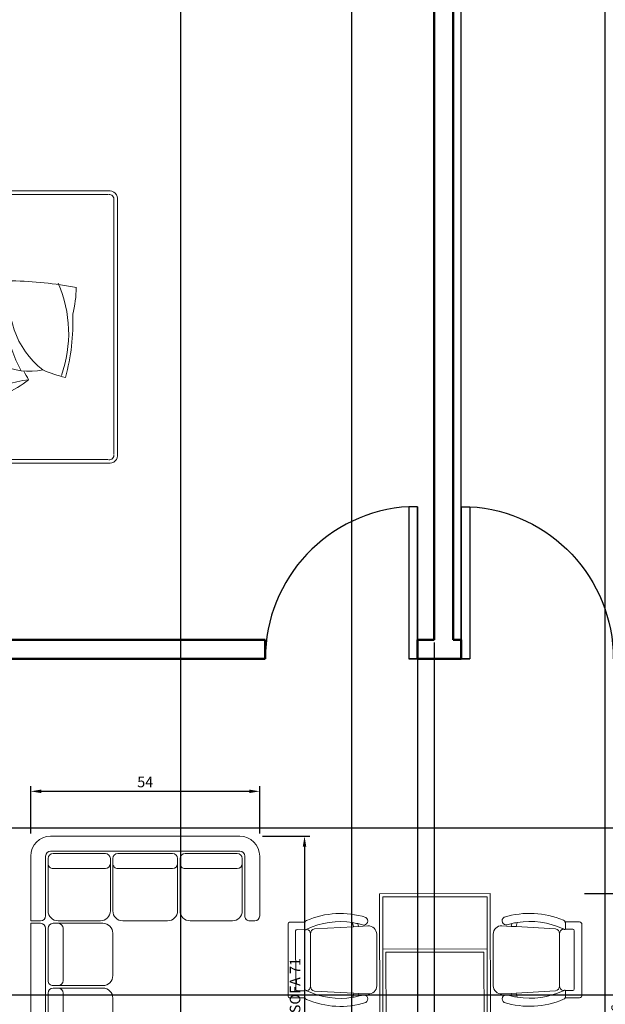
# Model space of a CAD drawing. Units: inches. Extents: x 907 to 2409, y 377 to 1163.
# Tile 5 of 9: x 1058 to 1197, y 687 to 920. Entities that reach past the tile are written whole.
import ezdxf

# ---------------------------------------------------------------- set-up
doc = ezdxf.new("R2010")
doc.units = ezdxf.units.IN
for name, color, linetype, lineweight in [('A-ANNO-DIMS', 2, 'Continuous', 18), ('A-DOOR', 3, 'Continuous', 25), ('A-FURN', 8, 'Continuous', 18), ('A-WALL', 7, 'Continuous', 50)]:
    doc.layers.add(name, color=color, linetype=linetype, lineweight=lineweight)
doc.styles.get("Standard").update_dxf_attribs({"font": 'arial.ttf'})
doc.dimstyles.new('ISO-25', dxfattribs={"dimtxt": 2.5, "dimasz": 2.5, "dimexe": 1.25, "dimexo": 0.625, "dimtad": 1, "dimtxsty": 'Standard', "dimcen": 2.5, "dimadec": 0, "dimazin": 0, "dimtfac": 1, "dimtmove": 0, "dimatfit": 3, "dimfxl": 1, "dimarcsym": 0})

# ---------------------------------------------------------------- blocks, each defined once
blk = doc.blocks.new('A$C356F0359')
for p, q in [((0.4398, 1.9801), (0.0598, 1.9801)), ((0.4398, 1.9601), (0.0598, 1.9601)), ((0.5489, 2), (2.0492, 2)), ((0.5489, 1.9489), (0.5489, 2)), ((2.0492, 1.9489), (2.0492, 2)), ((2.5283, 1.9801), (2.1483, 1.9801)), ((2.5283, 1.9601), (2.1483, 1.9601)), ((-0.0002, 1.9201), (-0.0002, 1.5401)), ((0.0198, 1.9201), (0.0198, 1.5401)), ((0.4798, 1.5401), (0.4798, 1.9201)), ((0.4998, 1.5401), (0.4998, 1.9201)), ((2.0492, 1.9489), (0.5489, 1.9489)), ((1.998, 1.9289), (0.6001, 1.9289)), ((2.0883, 1.9201), (2.0883, 1.5401)), ((2.1083, 1.9201), (2.1083, 1.5401)), ((2.5683, 1.5401), (2.5683, 1.9201)), ((2.5883, 1.5401), (2.5883, 1.9201)), ((0.1539, 1.5681), (0.1539, 1.8777)), ((0.2725, 1.8879), (0.2702, 1.8856)), ((0.2702, 1.8856), (0.2702, 1.7279)), ((0.2725, 1.8879), (0.4531, 1.8879)), ((0.3913, 1.8753), (0.277, 1.8753)), ((0.277, 1.8753), (0.277, 1.8147)), ((0.3913, 1.8147), (0.3913, 1.8753)), ((0.4016, 1.8787), (0.4062, 1.8845)), ((0.4016, 1.7404), (0.4016, 1.8787)), ((0.4062, 1.881), (0.405, 1.8765)), ((0.405, 1.8765), (0.4153, 1.8662)), ((0.405, 1.8765), (0.405, 1.8456)), ((0.405, 1.8456), (0.4073, 1.8399)), ((0.4062, 1.8845), (0.4405, 1.8845)), ((0.4108, 1.8833), (0.4062, 1.881)), ((0.4108, 1.8833), (0.4382, 1.8833)), ((0.4165, 1.8685), (0.4108, 1.8833)), ((0.4153, 1.8662), (0.4165, 1.8685)), ((0.4153, 1.8147), (0.4153, 1.8662)), ((0.4325, 1.8685), (0.4165, 1.8685)), ((0.4325, 1.8685), (0.4382, 1.8833)), ((0.4336, 1.8662), (0.4325, 1.8685)), ((0.4439, 1.8765), (0.4336, 1.8662)), ((0.4336, 1.8147), (0.4336, 1.8662)), ((0.4382, 1.8833), (0.4428, 1.881)), ((0.4405, 1.8845), (0.4462, 1.8787)), ((0.4439, 1.8456), (0.4416, 1.8399)), ((0.4428, 1.881), (0.4439, 1.8765)), ((0.4439, 1.8765), (0.4439, 1.8456)), ((0.4462, 1.8787), (0.4462, 1.7416)), ((0.4531, 1.8879), (0.4553, 1.8856)), ((0.4553, 1.8856), (0.4553, 1.7279)), ((0.5489, 1.8977), (0.5489, 0.0512)), ((0.5689, 1.8977), (0.5689, 0.0512)), ((2.0292, 0.0512), (2.0292, 1.8977)), ((2.0492, 0.0512), (2.0492, 1.8977)), ((2.3306, 1.5822), (2.3306, 1.8917)), ((0.277, 1.8147), (0.3913, 1.8147)), ((0.3913, 1.8125), (0.2816, 1.8125)), ((0.2816, 1.8125), (0.2816, 1.801)), ((0.2816, 1.801), (0.3913, 1.801)), ((0.2907, 1.8125), (0.2907, 1.801)), ((0.2999, 1.8125), (0.2999, 1.801)), ((0.309, 1.8125), (0.309, 1.801)), ((0.3182, 1.8125), (0.3182, 1.801)), ((0.3273, 1.8125), (0.3273, 1.801)), ((0.3365, 1.8125), (0.3365, 1.801)), ((0.3913, 1.801), (0.3913, 1.8125)), ((0.4073, 1.8399), (0.4108, 1.8342)), ((0.4108, 1.8342), (0.4119, 1.8262)), ((0.4108, 1.785), (0.4119, 1.793)), ((0.4119, 1.8262), (0.4119, 1.8147)), ((0.4119, 1.793), (0.4119, 1.8147)), ((0.4153, 1.8147), (0.4153, 1.753)), ((0.4336, 1.8147), (0.4336, 1.753)), ((0.4382, 1.8342), (0.4371, 1.8262)), ((0.4371, 1.8262), (0.4371, 1.8147)), ((0.4371, 1.793), (0.4371, 1.8147)), ((0.4382, 1.785), (0.4371, 1.793)), ((0.4416, 1.8399), (0.4382, 1.8342)), ((0.277, 1.7885), (0.277, 1.7679)), ((0.3445, 1.7885), (0.277, 1.7885)), ((0.277, 1.7679), (0.3445, 1.7679)), ((0.2782, 1.7622), (0.2782, 1.7576)), ((0.2896, 1.7622), (0.2782, 1.7622)), ((0.2782, 1.7576), (0.2896, 1.7576)), ((0.2782, 1.745), (0.2896, 1.745)), ((0.2782, 1.7382), (0.2782, 1.745)), ((0.2896, 1.7382), (0.2782, 1.7382)), ((0.2885, 1.7862), (0.2885, 1.7827)), ((0.2919, 1.7862), (0.2885, 1.7862)), ((0.2885, 1.7827), (0.2919, 1.7827)), ((0.2919, 1.7736), (0.2885, 1.7736)), ((0.2885, 1.7736), (0.2885, 1.7702)), ((0.2885, 1.7702), (0.2919, 1.7702)), ((0.2896, 1.7576), (0.2896, 1.7622)), ((0.2896, 1.745), (0.2896, 1.7382)), ((0.2919, 1.7827), (0.2919, 1.7862)), ((0.2919, 1.7702), (0.2919, 1.7736)), ((0.2942, 1.7622), (0.2942, 1.7576)), ((0.3056, 1.7622), (0.2942, 1.7622)), ((0.2942, 1.7576), (0.3056, 1.7576)), ((0.2942, 1.745), (0.3056, 1.745)), ((0.2942, 1.7382), (0.2942, 1.745)), ((0.3056, 1.7382), (0.2942, 1.7382)), ((0.3056, 1.7576), (0.3056, 1.7622)), ((0.3056, 1.745), (0.3056, 1.7382)), ((0.3125, 1.7862), (0.309, 1.7862)), ((0.309, 1.7862), (0.309, 1.7827)), ((0.309, 1.7827), (0.3125, 1.7827)), ((0.3125, 1.7736), (0.309, 1.7736)), ((0.309, 1.7736), (0.309, 1.7702)), ((0.309, 1.7702), (0.3125, 1.7702)), ((0.3102, 1.7622), (0.3102, 1.7576)), ((0.3216, 1.7622), (0.3102, 1.7622)), ((0.3102, 1.7576), (0.3216, 1.7576)), ((0.3102, 1.745), (0.3216, 1.745)), ((0.3102, 1.7382), (0.3102, 1.745)), ((0.3216, 1.7382), (0.3102, 1.7382)), ((0.3125, 1.7827), (0.3125, 1.7862)), ((0.3125, 1.7702), (0.3125, 1.7736)), ((0.3216, 1.7576), (0.3216, 1.7622)), ((0.3216, 1.745), (0.3216, 1.7382)), ((0.3376, 1.7622), (0.3262, 1.7622)), ((0.3262, 1.7622), (0.3262, 1.7576)), ((0.3262, 1.7576), (0.3376, 1.7576)), ((0.3262, 1.7382), (0.3262, 1.745)), ((0.3262, 1.745), (0.3376, 1.745)), ((0.3376, 1.7382), (0.3262, 1.7382)), ((0.333, 1.7862), (0.3296, 1.7862)), ((0.3296, 1.7862), (0.3296, 1.7827)), ((0.3296, 1.7827), (0.333, 1.7827)), ((0.333, 1.7736), (0.3296, 1.7736)), ((0.3296, 1.7736), (0.3296, 1.7702)), ((0.3296, 1.7702), (0.333, 1.7702)), ((0.333, 1.7827), (0.333, 1.7862)), ((0.333, 1.7702), (0.333, 1.7736)), ((0.3376, 1.7576), (0.3376, 1.7622)), ((0.3376, 1.745), (0.3376, 1.7382)), ((0.3445, 1.7679), (0.3445, 1.7885)), ((0.3548, 1.7759), (0.3548, 1.7827)), ((0.3548, 1.7827), (0.3639, 1.7827)), ((0.3639, 1.7759), (0.3548, 1.7759)), ((0.3548, 1.7633), (0.3548, 1.7702)), ((0.3548, 1.7702), (0.3639, 1.7702)), ((0.3639, 1.7633), (0.3548, 1.7633)), ((0.3548, 1.7564), (0.3639, 1.7564)), ((0.3548, 1.7496), (0.3548, 1.7564)), ((0.3639, 1.7496), (0.3548, 1.7496)), ((0.3548, 1.737), (0.3548, 1.7439)), ((0.3548, 1.7439), (0.3639, 1.7439)), ((0.3639, 1.737), (0.3548, 1.737)), ((0.3639, 1.7827), (0.3639, 1.7759)), ((0.3639, 1.7702), (0.3639, 1.7633)), ((0.3639, 1.7564), (0.3639, 1.7496)), ((0.3639, 1.7439), (0.3639, 1.737)), ((0.3685, 1.7827), (0.3776, 1.7827)), ((0.3685, 1.7759), (0.3685, 1.7827)), ((0.3776, 1.7759), (0.3685, 1.7759)), ((0.3685, 1.7633), (0.3685, 1.7702)), ((0.3685, 1.7702), (0.3776, 1.7702)), ((0.3776, 1.7633), (0.3685, 1.7633)), ((0.3685, 1.7564), (0.3776, 1.7564)), ((0.3685, 1.7496), (0.3685, 1.7564)), ((0.3776, 1.7496), (0.3685, 1.7496)), ((0.3685, 1.737), (0.3685, 1.7439)), ((0.3685, 1.7439), (0.3776, 1.7439)), ((0.3776, 1.737), (0.3685, 1.737)), ((0.3776, 1.7827), (0.3776, 1.7759)), ((0.3776, 1.7702), (0.3776, 1.7633)), ((0.3776, 1.7564), (0.3776, 1.7496)), ((0.3776, 1.7439), (0.3776, 1.737)), ((0.3822, 1.7759), (0.3822, 1.7827)), ((0.3822, 1.7827), (0.3913, 1.7827)), ((0.3913, 1.7759), (0.3822, 1.7759)), ((0.3822, 1.7633), (0.3822, 1.7702)), ((0.3822, 1.7702), (0.3913, 1.7702)), ((0.3913, 1.7633), (0.3822, 1.7633)), ((0.3822, 1.7576), (0.3913, 1.7576)), ((0.3822, 1.7507), (0.3822, 1.7576)), ((0.3913, 1.7507), (0.3822, 1.7507)), ((0.3822, 1.7439), (0.3913, 1.7439)), ((0.3822, 1.737), (0.3822, 1.7439)), ((0.3913, 1.737), (0.3822, 1.737)), ((0.3913, 1.7827), (0.3913, 1.7759)), ((0.3913, 1.7702), (0.3913, 1.7633)), ((0.3913, 1.7576), (0.3913, 1.7507)), ((0.3913, 1.7439), (0.3913, 1.737)), ((0.4073, 1.7347), (0.4016, 1.7404)), ((0.405, 1.7736), (0.4073, 1.7793)), ((0.405, 1.7427), (0.405, 1.7736)), ((0.405, 1.7427), (0.4153, 1.753)), ((0.4062, 1.7382), (0.405, 1.7427)), ((0.4108, 1.7359), (0.4062, 1.7382)), ((0.4073, 1.7793), (0.4108, 1.785)), ((0.4165, 1.7507), (0.4108, 1.7359)), ((0.4108, 1.7359), (0.4234, 1.7359)), ((0.4153, 1.753), (0.4165, 1.7507)), ((0.4325, 1.7507), (0.4165, 1.7507)), ((0.4233, 1.7393), (0.4235, 1.7294)), ((0.4268, 1.7393), (0.4233, 1.7393)), ((0.4274, 1.7301), (0.4268, 1.7393)), ((0.427, 1.7359), (0.4382, 1.7359)), ((0.4336, 1.753), (0.4325, 1.7507)), ((0.4325, 1.7507), (0.4382, 1.7359)), ((0.4439, 1.7427), (0.4336, 1.753)), ((0.4416, 1.7793), (0.4382, 1.785)), ((0.4382, 1.7359), (0.4428, 1.7382)), ((0.4462, 1.7416), (0.4405, 1.7347)), ((0.4439, 1.7736), (0.4416, 1.7793)), ((0.4428, 1.7382), (0.4439, 1.7427)), ((0.4439, 1.7427), (0.4439, 1.7736)), ((0.4622, 1.7459), (0.4553, 1.7484)), ((0.4553, 1.7439), (0.4604, 1.7425)), ((0.4604, 1.7425), (0.465, 1.7388)), ((0.4654, 1.7427), (0.4622, 1.7459)), ((0.465, 1.7388), (0.4662, 1.7372)), ((0.4678, 1.7405), (0.4654, 1.7427)), ((0.4662, 1.7372), (0.4686, 1.7374)), ((0.4686, 1.7374), (0.4662, 1.735)), ((0.4721, 1.7421), (0.4678, 1.7405)), ((0.4741, 1.7401), (0.4721, 1.7421)), ((0.4725, 1.7366), (0.4741, 1.7401)), ((0.4753, 1.7388), (0.4725, 1.7366)), ((0.4783, 1.7356), (0.4753, 1.7388)), ((2.4819, 1.7366), (2.1818, 1.7366)), ((0.3052, 1.7226), (0.0051, 1.7226)), ((0.2702, 1.7279), (0.2725, 1.7256)), ((0.4244, 1.7256), (0.2725, 1.7256)), ((0.4234, 1.7347), (0.4073, 1.7347)), ((0.4235, 1.7294), (0.4263, 1.7179)), ((0.4263, 1.7179), (0.429, 1.707)), ((0.427, 1.697), (0.4265, 1.6915)), ((0.4265, 1.6915), (0.4332, 1.6903)), ((0.4332, 1.6903), (0.4267, 1.6864)), ((0.4267, 1.6864), (0.4272, 1.6801)), ((0.4295, 1.6996), (0.427, 1.697)), ((0.4405, 1.7347), (0.4271, 1.7347)), ((0.429, 1.7227), (0.4274, 1.7301)), ((0.4531, 1.7256), (0.4284, 1.7256)), ((0.429, 1.707), (0.4288, 1.701)), ((0.4288, 1.701), (0.4295, 1.6996)), ((0.4318, 1.7119), (0.429, 1.7227)), ((0.4325, 1.7063), (0.4318, 1.7119)), ((0.4323, 1.7003), (0.4325, 1.7063)), ((0.4364, 1.6973), (0.4323, 1.7003)), ((0.4355, 1.6919), (0.4364, 1.6973)), ((0.4367, 1.6774), (0.4355, 1.6919)), ((0.4553, 1.7279), (0.4531, 1.7256)), ((0.4662, 1.735), (0.4755, 1.7268)), ((0.4755, 1.7268), (0.4906, 1.7139)), ((0.4759, 1.729), (0.4783, 1.7356)), ((0.4821, 1.7322), (0.4759, 1.729)), ((0.4874, 1.7272), (0.4821, 1.7322)), ((0.4862, 1.7199), (0.4874, 1.7272)), ((0.4914, 1.7231), (0.4862, 1.7199)), ((0.4908, 1.7135), (0.4984, 1.6917)), ((0.4958, 1.7185), (0.4914, 1.7231)), ((0.494, 1.7135), (0.4958, 1.7185)), ((0.501, 1.7142), (0.494, 1.7135)), ((0.4984, 1.6917), (0.4952, 1.6744)), ((0.4964, 1.7047), (0.5031, 1.7072)), ((0.5038, 1.7049), (0.4964, 1.7047)), ((0.5005, 1.695), (0.5054, 1.6996)), ((0.5068, 1.695), (0.5005, 1.695)), ((0.5008, 1.6871), (0.5079, 1.6892)), ((0.5068, 1.6836), (0.5008, 1.6871)), ((0.5031, 1.7072), (0.501, 1.7142)), ((0.5054, 1.6996), (0.5038, 1.7049)), ((0.5058, 1.679), (0.5068, 1.6836)), ((0.5079, 1.6892), (0.5068, 1.695)), ((0.4272, 1.6801), (0.4346, 1.6794)), ((0.4346, 1.6794), (0.4281, 1.6744)), ((0.4281, 1.6744), (0.4311, 1.669)), ((0.4311, 1.669), (0.4381, 1.6704)), ((0.4381, 1.6704), (0.4348, 1.6639)), ((0.4348, 1.6639), (0.4383, 1.6598)), ((0.4455, 1.6663), (0.4367, 1.6774)), ((0.4383, 1.6598), (0.4436, 1.6637)), ((0.4436, 1.6637), (0.4427, 1.6575)), ((0.4427, 1.6575), (0.4471, 1.6547)), ((0.4577, 1.6598), (0.4455, 1.6663)), ((0.4471, 1.6547), (0.4526, 1.6593)), ((0.4526, 1.6593), (0.4519, 1.6517)), ((0.4519, 1.6517), (0.4568, 1.6503)), ((0.4568, 1.6503), (0.4598, 1.6565)), ((0.4716, 1.6586), (0.4577, 1.6598)), ((0.4598, 1.6565), (0.4626, 1.6503)), ((0.4626, 1.6503), (0.4665, 1.6498)), ((0.4665, 1.6498), (0.4681, 1.6565)), ((0.4681, 1.6565), (0.4707, 1.6491)), ((0.4707, 1.6491), (0.4751, 1.6503)), ((0.485, 1.6644), (0.4716, 1.6586)), ((0.4751, 1.6503), (0.4753, 1.6565)), ((0.4753, 1.6565), (0.4806, 1.6519)), ((0.4806, 1.6519), (0.4843, 1.6538)), ((0.4843, 1.6538), (0.4836, 1.6607)), ((0.4836, 1.6607), (0.4885, 1.6547)), ((0.4952, 1.6744), (0.485, 1.6644)), ((0.4885, 1.6547), (0.4922, 1.6579)), ((0.4922, 1.6579), (0.4894, 1.6642)), ((0.4894, 1.6642), (0.4959, 1.6614)), ((0.4957, 1.6704), (0.5024, 1.6683)), ((0.4989, 1.6642), (0.4957, 1.6704)), ((0.4959, 1.6614), (0.4989, 1.6642)), ((0.5042, 1.673), (0.4987, 1.6792)), ((0.4987, 1.6792), (0.5058, 1.679)), ((0.5024, 1.6683), (0.5042, 1.673)), ((0.0598, 1.5001), (0.4398, 1.5001)), ((0.0598, 1.4801), (0.4398, 1.4801)), ((2.1483, 1.5001), (2.5283, 1.5001)), ((2.1483, 1.4801), (2.5283, 1.4801)), ((0.6001, 0.02), (1.998, 0.02)), ((0.6001, 0), (1.998, 0))]:
    blk.add_line(p, q)
at = {"linetype": 'ByBlock'}
for p, q in [((0.6001, 1.9147), (1.282, 1.9147)), ((0.6001, 1.6759), (0.6001, 1.9147)), ((1.282, 1.9147), (1.282, 1.6759)), ((1.3161, 1.9147), (1.998, 1.9147)), ((1.3161, 1.6759), (1.3161, 1.9147)), ((1.998, 1.9147), (1.998, 1.6759)), ((1.0687, 1.6418), (0.5489, 1.6418)), ((1.282, 1.6759), (0.6001, 1.6759)), ((1.998, 1.6759), (1.3161, 1.6759)), ((1.4185, 1.5053), (0.5489, 1.5053))]:
    blk.add_line(p, q, dxfattribs=at)
for centre in [(2.3306, 1.7366), (0.1539, 1.7226)]:
    blk.add_circle(centre, 0.12, dxfattribs=at)
for centre in [(2.3306, 1.7366), (0.1539, 1.7226)]:
    blk.add_circle(centre, 0.06)
for centre, radius, start, end in [((0.0598, 1.9201), 0.06, 90, 180), ((0.0598, 1.9201), 0.04, 90, 180), ((0.4398, 1.9201), 0.06, 0, 90), ((0.4398, 1.9201), 0.04, 0, 90), ((2.1483, 1.9201), 0.06, 90, 180), ((2.1483, 1.9201), 0.04, 90, 180), ((2.5283, 1.9201), 0.06, 0, 90), ((2.5283, 1.9201), 0.04, 0, 90), ((0.6001, 1.8977), 0.0512, 90, 180), ((0.6001, 1.8977), 0.0312, 90, 180), ((1.998, 1.8977), 0.0512, 0, 90), ((1.998, 1.8977), 0.0312, 0, 90), ((0.0598, 1.5401), 0.06, 180, 270), ((0.0598, 1.5401), 0.04, 180, 270), ((0.4398, 1.5401), 0.04, 270, 0), ((0.4398, 1.5401), 0.06, 270, 0), ((2.1483, 1.5401), 0.06, 180, 270), ((2.1483, 1.5401), 0.04, 180, 270), ((2.5283, 1.5401), 0.06, 270, 0), ((2.5283, 1.5401), 0.04, 270, 0), ((1.1471, 0.7332), 0.3575, 102.4782, 140.4625), ((1.9086, 1.3124), 0.8697, 195.336, 226.4193), ((0.3249, 0.4335), 0.9879, 28.4971, 41.0566), ((0.9965, 0.4273), 0.548, 103.2034, 117.0362), ((1.6529, 1.7059), 1.0798, 223.6306, 251.4288), ((0.4451, 0.4375), 0.5655, 5.3391, 57.6895), ((0.4517, 0.5274), 0.4879, 10.6986, 52.6864), ((1.8195, 1.3719), 1.1652, 203.0642, 220.3209), ((0.5617, 0.4344), 0.7874, 18.3527, 36.6851), ((-0.021, 2.4319), 2.1977, 305.2966, 307.2418), ((1.5949, 0.9312), 0.734, 205.259, 216.9351), ((1.4135, 0.487), 0.3575, 154.0418, 192.0262), ((1.3641, 0.0041), 0.6085, 71.81, 120.1351), ((1.1372, -0.3434), 0.9879, 80.0607, 92.6202), ((1.2836, -0.1573), 0.7874, 69.9163, 88.2487), ((1.44, 0.1186), 0.4774, 76.1849, 142.0017), ((-0.6432, 0.628), 2.1977, 349.4884, 358.8054), ((-0.021, 2.4319), 2.1977, 297.9248, 299.3793), ((1.5595, 0.1789), 0.548, 154.767, 168.5998), ((1.2647, 0.9578), 0.6885, 250.2936, 293.6414), ((1.3312, 1.4107), 1.1652, 254.6278, 271.8845), ((1.5368, 0.9609), 0.734, 256.8226, 268.4988), ((0.5943, 0.0454), 0.0458, 172.7599, 277.2401), ((0.5943, 0.0454), 0.0258, 172.7599, 277.2401), ((2.0038, 0.0454), 0.0458, 262.7599, 7.2401), ((2.0038, 0.0454), 0.0258, 262.7599, 7.2401)]:
    blk.add_arc(centre, radius, start, end)
for centre, radius, start, end in [((0.1906, 1.7953), 0.4265, 343.7398, 16.2602), ((1.6914, 1.7953), 0.4265, 163.7398, 196.2602), ((0.9067, 1.7953), 0.4265, 343.7398, 16.2602), ((2.4075, 1.7953), 0.4265, 163.7398, 196.2602), ((0.9303, 0.657), 0.9853, 61.4328, 88.1261), ((1.0826, 0.5712), 1.0706, 72.1966, 90.7418), ((2.1368, 4.5996), 3.0955, 256.4201, 268.3789), ((2.0056, 2.7745), 1.3903, 244.2427, 271.7984)]:
    blk.add_arc(centre, radius, start, end, dxfattribs=at)
blk = doc.blocks.new('A$C2AFA021D')
for p, q in [((0.8, 2.3), (0.2, 2.3)), ((0.85, 2.2), (0.85, 2.25)), ((0, 2.1), (0, 0.2)), ((0.15, 0.2), (0.15, 2.1)), ((0.2, 2.15), (0.8, 2.15)), ((0.225, 2.125), (0.275, 2.125)), ((0.75, 2.125), (0.275, 2.125)), ((0.175, 1.55), (0.175, 2.075)), ((0.325, 2.075), (0.325, 1.55)), ((0.85, 1.6), (0.85, 2.025)), ((0.275, 1.5), (0.225, 1.5)), ((0.275, 1.5), (0.75, 1.5)), ((0.175, 0.875), (0.175, 1.425)), ((0.225, 1.475), (0.275, 1.475)), ((0.75, 1.475), (0.275, 1.475)), ((0.325, 1.425), (0.325, 0.875)), ((0.85, 0.925), (0.85, 1.375)), ((0.275, 0.825), (0.225, 0.825)), ((0.225, 0.8), (0.275, 0.8)), ((0.275, 0.825), (0.75, 0.825)), ((0.75, 0.8), (0.275, 0.8)), ((0.975, 0.825), (1.4, 0.825)), ((1.625, 0.825), (2.075, 0.825)), ((2.3, 0.825), (2.725, 0.825)), ((2.9, 0.825), (2.95, 0.825)), ((0.175, 0.225), (0.175, 0.75)), ((0.325, 0.75), (0.325, 0.225)), ((0.85, 0.275), (0.85, 0.7)), ((0.875, 0.275), (0.875, 0.725)), ((1.5, 0.725), (1.5, 0.275)), ((1.525, 0.275), (1.525, 0.725)), ((2.175, 0.725), (2.175, 0.275)), ((2.2, 0.275), (2.2, 0.725)), ((2.825, 0.725), (2.825, 0.275)), ((2.85, 0.2), (2.85, 0.775)), ((3, 0.775), (3, 0.2)), ((1.45, 0.325), (0.925, 0.325)), ((2.125, 0.325), (1.575, 0.325)), ((2.775, 0.325), (2.25, 0.325)), ((0.875, 0.275), (0.875, 0.225)), ((1.5, 0.225), (1.5, 0.275)), ((1.525, 0.275), (1.525, 0.225)), ((2.175, 0.225), (2.175, 0.275)), ((2.2, 0.275), (2.2, 0.225)), ((2.825, 0.225), (2.825, 0.275)), ((0.8, 0.15), (0.2, 0.15)), ((0.275, 0.175), (0.225, 0.175)), ((0.275, 0.175), (0.75, 0.175)), ((0.85, 0), (0.85, 0.1)), ((0.875, 0.1), (0.875, 0)), ((0.925, 0.175), (1.45, 0.175)), ((0.925, 0.15), (2.8, 0.15)), ((1.575, 0.175), (2.125, 0.175)), ((2.25, 0.175), (2.775, 0.175)), ((0.2, 0), (0.85, 0)), ((2.8, 0), (0.875, 0))]:
    blk.add_line(p, q)
for centre, radius, start, end in [((0.2, 2.1), 0.2, 90, 180), ((0.8, 2.25), 0.05, 0, 90), ((0.8, 2.2), 0.05, 270, 0), ((0.2, 2.1), 0.05, 90, 180), ((0.225, 2.075), 0.05, 90, 180), ((0.275, 2.075), 0.05, 0, 90), ((0.75, 2.025), 0.1, 0, 90), ((0.75, 1.6), 0.1, 270, 0), ((0.225, 1.55), 0.05, 180, 270), ((0.275, 1.55), 0.05, 270, 0), ((0.225, 1.425), 0.05, 90, 180), ((0.275, 1.425), 0.05, 0, 90), ((0.75, 1.375), 0.1, 360, 90), ((0.75, 0.925), 0.1, 270, 0), ((0.225, 0.875), 0.05, 180, 270), ((0.225, 0.75), 0.05, 90, 180), ((0.275, 0.875), 0.05, 270, 0), ((0.275, 0.75), 0.05, 0, 90), ((0.75, 0.7), 0.1, 0, 90), ((0.975, 0.725), 0.1, 90, 180), ((1.4, 0.725), 0.1, 0, 90), ((1.625, 0.725), 0.1, 90, 180), ((2.075, 0.725), 0.1, 0, 90), ((2.3, 0.725), 0.1, 90, 180), ((2.725, 0.725), 0.1, 0, 90), ((2.9, 0.775), 0.05, 90, 180), ((2.95, 0.775), 0.05, 0, 90), ((0.925, 0.275), 0.05, 90, 180), ((1.45, 0.275), 0.05, 360, 90), ((1.575, 0.275), 0.05, 90, 180), ((2.125, 0.275), 0.05, 360, 90), ((2.25, 0.275), 0.05, 90, 180), ((2.775, 0.275), 0.05, 360, 90), ((0.2, 0.2), 0.2, 180, 270), ((0.2, 0.2), 0.05, 180, 270), ((0.225, 0.225), 0.05, 180, 270), ((0.275, 0.225), 0.05, 270, 0), ((0.75, 0.275), 0.1, 270, 0), ((0.925, 0.225), 0.05, 180, 270), ((1.45, 0.225), 0.05, 270, 0), ((1.575, 0.225), 0.05, 180, 270), ((2.125, 0.225), 0.05, 270, 0), ((2.25, 0.225), 0.05, 180, 270), ((2.775, 0.225), 0.05, 270, 0), ((2.8, 0.2), 0.2, 270, 0), ((2.8, 0.2), 0.05, 270, 0), ((0.8, 0.1), 0.05, 0, 90), ((0.925, 0.1), 0.05, 90, 180)]:
    blk.add_arc(centre, radius, start, end)
blk = doc.blocks.new('A$C7D96336B')
for p, q in [((280, 0.2), (-280, -0.2)), ((280.8, -1199.8), (280, 0.2)), ((-280, -0.2), (-279.2, -1200.2)), ((264, -15.8), (-264, -16.2)), ((-264, -16.2), (-263.2, -1184.2)), ((264.8, -1183.8), (264, -15.8)), ((-658.1, -143.4), (-730.7, -143.6)), ((-659.8, -143.4), (-659.7, -178.7)), ((-416.5, -146.3), (-411.5, -167.3)), ((416.7, -145.7), (411.7, -166.7)), ((658.3, -142.5), (730.9, -142.6)), ((659.9, -142.6), (659.9, -177.8)), ((-742.8, -515.1), (-743.2, -156.2)), ((-704.9, -188.8), (-704.6, -482.3)), ((-659.3, -180.3), (-696.6, -180.5)), ((-411.5, -167.3), (-609.1, -178.7)), ((-386.1, -165.8), (-411.5, -167.3)), ((-389.5, -151.7), (-386.1, -165.8)), ((-338.9, -163.1), (-386.1, -165.8)), ((339.1, -162.6), (386.3, -165.3)), ((389.7, -151.1), (386.3, -165.3)), ((386.3, -165.3), (411.7, -166.7)), ((411.7, -166.7), (609.3, -177.8)), ((659.5, -179.5), (696.9, -179.5)), ((705.2, -187.9), (705.3, -481.4)), ((743.5, -514.1), (743.4, -155.2)), ((-629.9, -467.6), (-630.2, -203.4)), ((-294.5, -465.7), (-294.4, -204.7)), ((295.2, -465.3), (294.7, -204.3)), ((630.5, -466.8), (630.5, -202.5)), ((-263.8, -280.2), (264.2, -279.8)), ((-263.8, -280.2), (264.2, -279.8)), ((-263.4, -920.2), (-263.8, -280.2)), ((-247.8, -296.2), (248.2, -295.8)), ((-247.4, -904.2), (-247.8, -296.2)), ((248.2, -295.8), (248.6, -903.8)), ((264.2, -279.8), (264.6, -919.8)), ((-659, -490.7), (-696.3, -490.7)), ((-659.4, -522.3), (-659.3, -492.4)), ((-411.1, -503.3), (-608.7, -492.3)), ((411.8, -502.7), (609.4, -491.4)), ((659.6, -489.8), (697, -489.7)), ((660.1, -521.4), (660, -491.5)), ((-657.7, -527.6), (-730.3, -527.6)), ((-416.1, -524.3), (-411.1, -503.3)), ((-385.8, -504.7), (-411.1, -503.3)), ((-389.1, -518.8), (-385.8, -504.7)), ((-338.5, -507.3), (-385.8, -504.7)), ((339.2, -506.9), (386.5, -504.2)), ((386.5, -504.2), (411.8, -502.7)), ((389.8, -518.3), (386.5, -504.2)), ((416.8, -523.7), (411.8, -502.7)), ((658.4, -526.7), (731, -526.6)), ((-742.7, -688.4), (-742.6, -1047.3)), ((-657.6, -675.8), (-730.2, -675.9)), ((-659.3, -681), (-659.2, -711)), ((-416, -678.8), (-411, -699.8)), ((-389, -684.2), (-385.6, -698.3)), ((-338.4, -695.6), (-385.6, -698.3)), ((339.3, -695.2), (386.6, -697.8)), ((389.9, -683.7), (386.6, -697.8)), ((416.9, -678.2), (411.9, -699.2)), ((658.5, -674.9), (731.1, -674.9)), ((660.2, -680.2), (660.2, -710.1)), ((743.6, -687.4), (744, -1046.3)), ((-704.4, -1014.6), (-704.5, -721.1)), ((-658.8, -712.7), (-696.2, -712.8)), ((-629.7, -735.7), (-629.6, -1000)), ((-411, -699.8), (-608.6, -711)), ((-385.6, -698.3), (-411, -699.8)), ((-294.4, -737.1), (-293.9, -998.2)), ((295.3, -736.7), (295.2, -997.8)), ((386.6, -697.8), (411.9, -699.2)), ((411.9, -699.2), (609.5, -710.2)), ((630.7, -734.9), (631, -999.1)), ((659.8, -711.8), (697.1, -711.8)), ((705.8, -1013.7), (705.5, -720.2)), ((264.6, -919.8), (-263.4, -920.2)), ((248.6, -903.8), (-247.4, -904.2)), ((-658.7, -1023), (-696.1, -1023)), ((-659.1, -1059.9), (-659.1, -1024.7)), ((-410.9, -1035.8), (-608.5, -1024.6)), ((-415.9, -1056.8), (-410.9, -1035.8)), ((-385.5, -1037.2), (-410.9, -1035.8)), ((-388.9, -1051.4), (-385.5, -1037.2)), ((-338.3, -1039.9), (-385.5, -1037.2)), ((339.7, -1039.4), (386.9, -1036.7)), ((386.9, -1036.7), (412.3, -1035.2)), ((390.3, -1050.8), (386.9, -1036.7)), ((412.3, -1035.2), (609.9, -1023.8)), ((417.3, -1056.2), (412.3, -1035.2)), ((660.1, -1022.1), (697.4, -1022)), ((660.6, -1059), (660.5, -1023.8)), ((-657.5, -1059.9), (-730.1, -1059.9)), ((658.9, -1059), (731.5, -1058.9)), ((-263.2, -1184.2), (264.8, -1183.8)), ((-279.2, -1200.2), (280.8, -1199.8))]:
    blk.add_line(p, q)
for centre, radius, start, end in [((-730.7, -156.1), 12.5, 141.7605, 180.1459), ((-730.7, -156.1), 12.5, 90.1463, 141.7605), ((-643.2, -151), 16.7, 153.004, 184.8567), ((-643.2, -151), 16.7, 113.3258, 153.004), ((-478.6, -532.7), 432.3, 72.7119, 113.3258), ((-479.1, -531.9), 390.7, 80.7703, 115.5809), ((-479.1, -531.9), 390.7, 76.7336, 80.7703), ((-360.6, -137.9), 20.8, 254.7795, 60.0186), ((360.7, -137.4), 20.8, 120.0589, 285.298), ((479.4, -532), 432.3, 66.7517, 107.3656), ((479.9, -531.2), 390.7, 99.3072, 103.3439), ((479.9, -531.2), 390.7, 64.4966, 99.3072), ((643.4, -150.1), 16.7, 27.0735, 66.7517), ((643.4, -150.1), 16.7, 355.2209, 27.0735), ((730.9, -155.1), 12.5, 38.317, 89.9312), ((730.9, -155.1), 12.5, 359.9316, 38.317), ((-696.6, -188.8), 8.33, 90.1463, 180.1463), ((-655.5, -178.6), 4.17, 180.1463, 296.5296), ((-479.1, -531.9), 390.7, 115.5809, 116.5296), ((-655.2, -203.4), 25, 0.1463, 72.8968), ((-605.2, -203.4), 25, 98.9209, 179.9714), ((-479.1, -531.9), 390.7, 73.1676, 76.7336), ((-336.5, -204.7), 41.7, 0.1463, 93.3068), ((336.7, -204.2), 41.7, 86.7707, 179.9312), ((479.9, -531.2), 390.7, 103.3439, 106.9099), ((605.5, -202.6), 25, 0.1061, 81.1566), ((655.5, -202.5), 25, 107.1807, 179.9312), ((479.9, -531.2), 390.7, 63.5479, 64.4966), ((655.7, -177.8), 4.17, 243.5479, 359.9312), ((696.9, -187.8), 8.33, 359.9312, 89.9312), ((-696.3, -482.3), 8.33, 179.9714, 269.9714), ((-655.2, -492.4), 4.17, 63.5881, 179.9714), ((-479.5, -138.8), 390.7, 243.5881, 244.5368), ((-654.9, -467.6), 25, 287.2209, 359.9714), ((-479.5, -138.8), 390.7, 244.5368, 279.3474), ((-604.9, -467.6), 25, 180.1463, 261.1967), ((-336.2, -465.7), 41.7, 266.8108, 359.9714), ((336.8, -465.3), 41.7, 180.1061, 273.2667), ((479.7, -138.1), 390.7, 260.7301, 295.5407), ((605.5, -466.7), 25, 278.8808, 359.9312), ((655.5, -466.7), 25, 180.1061, 252.8566), ((479.7, -138.1), 390.7, 295.5407, 296.4894), ((655.8, -491.5), 4.17, 0.1061, 116.4894), ((697, -481.4), 8.33, 270.1061, 0.1061), ((-730.3, -515.1), 12.5, 179.9717, 218.3572), ((-730.3, -515.1), 12.5, 218.3572, 269.9714), ((-642.9, -520), 16.7, 175.261, 207.1136), ((-642.9, -520), 16.7, 207.1136, 246.7919), ((-479.1, -138), 432.3, 246.7919, 287.4058), ((-479.5, -138.8), 390.7, 279.3474, 283.3841), ((-479.5, -138.8), 390.7, 283.3841, 286.9501), ((-360.2, -532.5), 20.8, 300.0991, 105.3382), ((360.9, -532), 20.8, 74.7393, 239.9785), ((479.2, -137.3), 432.3, 252.6717, 293.2857), ((479.7, -138.1), 390.7, 253.1274, 256.6934), ((479.7, -138.1), 390.7, 256.6934, 260.7301), ((643.6, -519.1), 16.7, 293.2857, 332.9639), ((643.6, -519.1), 16.7, 332.9639, 4.8165), ((731, -514.1), 12.5, 270.1061, 321.7203), ((731, -514.1), 12.5, 321.7203, 0.1058), ((-478.4, -1065.1), 432.3, 72.6717, 113.2857), ((479.9, -1064.5), 432.3, 66.7919, 107.4058), ((-730.2, -688.4), 12.5, 141.7203, 180.1058), ((-730.2, -688.4), 12.5, 90.1061, 141.7203), ((-642.7, -683.3), 16.7, 152.9639, 184.8165), ((-642.7, -683.3), 16.7, 113.2857, 152.9639), ((-478.9, -1064.3), 390.7, 80.7301, 115.5407), ((-478.9, -1064.3), 390.7, 76.6934, 80.7301), ((-478.9, -1064.3), 390.7, 73.1274, 76.6934), ((-360.1, -670.4), 20.8, 254.7393, 59.9785), ((-336, -737.2), 41.7, 0.1061, 93.2667), ((337, -736.8), 41.7, 86.8108, 179.9714), ((361, -670), 20.8, 120.0991, 285.3382), ((480.4, -1063.7), 390.7, 103.3841, 106.9501), ((480.4, -1063.7), 390.7, 99.3474, 103.3841), ((480.4, -1063.7), 390.7, 64.5368, 99.3474), ((643.7, -682.5), 16.7, 27.1136, 66.7919), ((643.7, -682.5), 16.7, 355.261, 27.1136), ((731.1, -687.4), 12.5, 38.3572, 89.9714), ((731.1, -687.4), 12.5, 359.9717, 38.3572), ((-696.1, -721.1), 8.33, 90.1061, 180.1061), ((-655, -711), 4.17, 180.1061, 296.4894), ((-478.9, -1064.3), 390.7, 115.5407, 116.4894), ((-654.7, -735.8), 25, 0.1061, 72.8566), ((-604.7, -735.7), 25, 98.8808, 179.9312), ((605.7, -734.9), 25, 0.1463, 81.1967), ((655.7, -734.9), 25, 107.2209, 179.9714), ((480.4, -1063.7), 390.7, 63.5881, 64.5368), ((656, -710.1), 4.17, 243.5881, 359.9714), ((697.1, -720.1), 8.33, 359.9714, 89.9714), ((-696.1, -1014.6), 8.33, 179.9312, 269.9312), ((-654.9, -1024.7), 4.17, 63.5479, 179.9312), ((-479.1, -671.2), 390.7, 243.5479, 244.4966), ((-654.6, -1000), 25, 287.1807, 359.9312), ((-479.1, -671.2), 390.7, 244.4966, 279.3072), ((-604.6, -999.9), 25, 180.1061, 261.1566), ((-479.1, -671.2), 390.7, 283.3439, 286.9099), ((-359.9, -1065.1), 20.8, 300.0589, 105.298), ((-335.9, -998.3), 41.7, 266.7707, 359.9312), ((337.3, -997.8), 41.7, 180.1463, 273.3068), ((361.4, -1064.6), 20.8, 74.7795, 240.0186), ((480, -670.6), 390.7, 253.1676, 256.7336), ((480, -670.6), 390.7, 260.7703, 295.5809), ((606, -999.1), 25, 278.9209, 359.9714), ((656, -999.1), 25, 180.1463, 252.8968), ((480, -670.6), 390.7, 295.5809, 296.5296), ((656.3, -1023.8), 4.17, 0.1463, 116.5296), ((697.4, -1013.7), 8.33, 270.1463, 0.1463), ((-730.1, -1047.4), 12.5, 179.9316, 218.317), ((-730.1, -1047.4), 12.5, 218.317, 269.9312), ((-642.6, -1052.4), 16.7, 175.2209, 207.0735), ((-642.6, -1052.4), 16.7, 207.0735, 246.7517), ((-478.6, -670.4), 432.3, 246.7517, 287.3656), ((-479.1, -671.2), 390.7, 279.3072, 283.3439), ((479.5, -669.8), 432.3, 252.7119, 293.3258), ((480, -670.6), 390.7, 256.7336, 260.7703), ((644, -1051.5), 16.7, 293.3258, 333.004), ((644, -1051.5), 16.7, 333.004, 4.8567), ((731.5, -1046.4), 12.5, 270.1463, 321.7605), ((731.5, -1046.4), 12.5, 321.7605, 0.1459)]:
    blk.add_arc(centre, radius, start, end)
blk = doc.blocks.new('DOOR-36IN')
for p, q in [((36, 36), (36, 0)), ((36, 0), (34, 0)), ((36, 0), (34, 0))]:
    blk.add_line(p, q)
blk.add_lwpolyline([(36, 36), (34, 36), (34, 0), (36, 0)], close=True)
blk.add_arc((36.06, 0), 36.06, 93.2732, 180)
blk = doc.blocks.new('*D53')
at = {"layer": 'A-ANNO-DIMS', "color": 0, "lineweight": -2, "transparency": 16777216}
for p, q in [((1115.67, 726.66), (1126.9, 726.66)), ((1125.65, 724.16), (1125.65, 658.44)), ((1115.67, 655.94), (1126.9, 655.94))]:
    blk.add_line(p, q, dxfattribs=at)
at = {"layer": 'A-ANNO-DIMS', "color": 0, "transparency": 16777216}
for points in [[(1125.24, 724.16), (1126.07, 724.16), (1125.65, 726.66)], [(1125.24, 658.44), (1126.07, 658.44), (1125.65, 655.94)]]:
    blk.add_solid(points, dxfattribs=at)
at = {"layer": 'Defpoints', "color": 0, "transparency": 16777216}
for p in [(1115.05, 726.66), (1115.05, 655.94), (1125.65, 655.94)]:
    blk.add_point(p, dxfattribs=at)
at = {"layer": 'A-ANNO-DIMS', "color": 0, "transparency": 16777216, "insert": (1123.74, 691.3), "char_height": 2.5, "attachment_point": 5, "rotation": 90}
blk.add_mtext('SOFA 71', dxfattribs=at)
blk = doc.blocks.new('*D54')
at = {"layer": 'A-ANNO-DIMS', "color": 0, "lineweight": -2, "transparency": 16777216}
for p, q in [((1060.83, 727.28), (1060.83, 738.52)), ((1063.33, 737.27), (1112.55, 737.27)), ((1115.05, 727.28), (1115.05, 738.52))]:
    blk.add_line(p, q, dxfattribs=at)
at = {"layer": 'A-ANNO-DIMS', "color": 0, "transparency": 16777216}
for points in [[(1063.33, 737.68), (1063.33, 736.85), (1060.83, 737.27)], [(1112.55, 737.68), (1112.55, 736.85), (1115.05, 737.27)]]:
    blk.add_solid(points, dxfattribs=at)
at = {"layer": 'Defpoints', "color": 0, "transparency": 16777216}
for p in [(1115.05, 737.27), (1060.83, 726.66), (1115.05, 726.66)]:
    blk.add_point(p, dxfattribs=at)
at = {"layer": 'A-ANNO-DIMS', "color": 0, "transparency": 16777216, "insert": (1087.94, 739.16), "char_height": 2.5, "attachment_point": 5}
blk.add_mtext('54', dxfattribs=at)
blk = doc.blocks.new('*D58')
at = {"layer": 'A-ANNO-DIMS', "color": 0, "lineweight": -2, "transparency": 16777216}
for p, q in [((1191.96, 713.06), (1203.02, 713.06)), ((1201.77, 659.4), (1201.77, 710.56)), ((1191.96, 656.9), (1203.02, 656.9))]:
    blk.add_line(p, q, dxfattribs=at)
at = {"layer": 'A-ANNO-DIMS', "color": 0, "transparency": 16777216}
for points in [[(1201.36, 710.56), (1202.19, 710.56), (1201.77, 713.06)], [(1201.36, 659.4), (1202.19, 659.4), (1201.77, 656.9)]]:
    blk.add_solid(points, dxfattribs=at)
at = {"layer": 'Defpoints', "color": 0, "transparency": 16777216}
for p in [(1191.34, 713.06), (1201.77, 713.06), (1191.34, 656.9)]:
    blk.add_point(p, dxfattribs=at)
at = {"layer": 'A-ANNO-DIMS', "color": 0, "transparency": 16777216, "insert": (1199.87, 684.98), "char_height": 2.5, "attachment_point": 5, "rotation": 90}
blk.add_mtext('56', dxfattribs=at)
blk = doc.blocks.new('*D59')
at = {"layer": 'A-ANNO-DIMS', "color": 0, "lineweight": -2, "transparency": 16777216}
for p, q in [((987.61, 773.75), (987.61, 1056.62)), ((1156.36, 773.75), (1156.36, 1056.62)), ((990.11, 1055.37), (1153.86, 1055.37))]:
    blk.add_line(p, q, dxfattribs=at)
at = {"layer": 'A-ANNO-DIMS', "color": 0, "transparency": 16777216}
for points in [[(990.11, 1055.79), (990.11, 1054.95), (987.61, 1055.37)], [(1153.86, 1055.79), (1153.86, 1054.95), (1156.36, 1055.37)]]:
    blk.add_solid(points, dxfattribs=at)
at = {"layer": 'Defpoints', "color": 0, "transparency": 16777216}
for p in [(1156.36, 1055.37), (987.61, 773.12), (1156.36, 773.12)]:
    blk.add_point(p, dxfattribs=at)
at = {"layer": 'A-ANNO-DIMS', "color": 0, "transparency": 16777216, "insert": (1071.99, 1057.27), "char_height": 2.5, "attachment_point": 5}
blk.add_mtext('168.75', dxfattribs=at)
blk = doc.blocks.new('*D61')
at = {"layer": 'A-ANNO-DIMS', "color": 0, "lineweight": -2, "transparency": 16777216}
for p, q in [((1052.86, 729.25), (1052.86, 1056.62)), ((1196.86, 727.25), (1196.86, 1056.62)), ((1055.36, 1055.37), (1194.36, 1055.37))]:
    blk.add_line(p, q, dxfattribs=at)
at = {"layer": 'A-ANNO-DIMS', "color": 0, "transparency": 16777216}
for points in [[(1055.36, 1055.79), (1055.36, 1054.95), (1052.86, 1055.37)], [(1194.36, 1055.79), (1194.36, 1054.95), (1196.86, 1055.37)]]:
    blk.add_solid(points, dxfattribs=at)
at = {"layer": 'Defpoints', "color": 0, "transparency": 16777216}
for p in [(1196.86, 1055.37), (1052.86, 728.62), (1196.86, 726.62)]:
    blk.add_point(p, dxfattribs=at)
at = {"layer": 'A-ANNO-DIMS', "color": 0, "transparency": 16777216, "insert": (1124.86, 1057.25), "char_height": 2.5, "attachment_point": 5}
blk.add_mtext('144', dxfattribs=at)
blk = doc.blocks.new('*D62')
at = {"layer": 'A-ANNO-DIMS', "color": 0, "lineweight": -2, "transparency": 16777216}
for p, q in [((987.61, 426.5), (987.61, 1056.62)), ((1096.36, 426.5), (1096.36, 1056.62)), ((990.11, 1055.37), (1093.86, 1055.37))]:
    blk.add_line(p, q, dxfattribs=at)
at = {"layer": 'A-ANNO-DIMS', "color": 0, "transparency": 16777216}
for points in [[(990.11, 1055.79), (990.11, 1054.95), (987.61, 1055.37)], [(1093.86, 1055.79), (1093.86, 1054.95), (1096.36, 1055.37)]]:
    blk.add_solid(points, dxfattribs=at)
at = {"layer": 'Defpoints', "color": 0, "transparency": 16777216}
for p in [(1096.36, 1055.37), (987.61, 425.87), (1096.36, 425.87)]:
    blk.add_point(p, dxfattribs=at)
at = {"layer": 'A-ANNO-DIMS', "color": 0, "transparency": 16777216, "insert": (1041.99, 1057.27), "char_height": 2.5, "attachment_point": 5}
blk.add_mtext('108.75', dxfattribs=at)
blk = doc.blocks.new('*D75')
at = {"layer": 'A-ANNO-DIMS', "color": 0, "lineweight": -2, "transparency": 16777216}
for p, q in [((1136.86, 613.25), (1136.86, 1056.62)), ((1196.86, 613.25), (1196.86, 1056.62)), ((1139.36, 1055.37), (1194.36, 1055.37))]:
    blk.add_line(p, q, dxfattribs=at)
at = {"layer": 'A-ANNO-DIMS', "color": 0, "transparency": 16777216}
for points in [[(1139.36, 1055.79), (1139.36, 1054.95), (1136.86, 1055.37)], [(1194.36, 1055.79), (1194.36, 1054.95), (1196.86, 1055.37)]]:
    blk.add_solid(points, dxfattribs=at)
at = {"layer": 'Defpoints', "color": 0, "transparency": 16777216}
for p in [(1196.86, 1055.37), (1136.86, 612.62), (1196.86, 612.62)]:
    blk.add_point(p, dxfattribs=at)
at = {"layer": 'A-ANNO-DIMS', "color": 0, "transparency": 16777216, "insert": (1166.86, 1057.27), "char_height": 2.5, "attachment_point": 5}
blk.add_mtext('60', dxfattribs=at)
blk = doc.blocks.new('*D81')
at = {"layer": 'A-ANNO-DIMS', "color": 0, "lineweight": -2, "transparency": 16777216}
for p, q in [((1053.49, 728.62), (1378.36, 728.62)), ((1377.11, 726.12), (1377.11, 691.62)), ((1048.99, 689.12), (1378.36, 689.12))]:
    blk.add_line(p, q, dxfattribs=at)
at = {"layer": 'A-ANNO-DIMS', "color": 0, "transparency": 16777216}
for points in [[(1376.7, 726.12), (1377.53, 726.12), (1377.11, 728.62)], [(1376.7, 691.62), (1377.53, 691.62), (1377.11, 689.12)]]:
    blk.add_solid(points, dxfattribs=at)
at = {"layer": 'Defpoints', "color": 0, "transparency": 16777216}
for p in [(1052.86, 728.62), (1048.36, 689.12), (1377.11, 689.12)]:
    blk.add_point(p, dxfattribs=at)
at = {"layer": 'A-ANNO-DIMS', "color": 0, "transparency": 16777216, "insert": (1375.21, 708.87), "char_height": 2.5, "attachment_point": 5, "rotation": 90}
blk.add_mtext('39.5', dxfattribs=at)
blk = doc.blocks.new('*D84')
at = {"layer": 'A-ANNO-DIMS', "color": 0, "lineweight": -2, "transparency": 16777216}
for p, q in [((1152.36, 772.5), (1152.36, 377.12)), ((1156.36, 772.5), (1156.36, 377.12)), ((1149.86, 378.37), (1147.36, 378.37)), ((1152.36, 378.37), (1156.36, 378.37)), ((1158.86, 378.37), (1161.36, 378.37))]:
    blk.add_line(p, q, dxfattribs=at)
at = {"layer": 'A-ANNO-DIMS', "color": 0, "transparency": 16777216}
for points in [[(1149.86, 378.79), (1149.86, 377.95), (1152.36, 378.37)], [(1158.86, 378.79), (1158.86, 377.95), (1156.36, 378.37)]]:
    blk.add_solid(points, dxfattribs=at)
at = {"layer": 'Defpoints', "color": 0, "transparency": 16777216}
for p in [(1152.36, 773.12), (1156.36, 773.12), (1156.36, 378.37)]:
    blk.add_point(p, dxfattribs=at)
at = {"layer": 'A-ANNO-DIMS', "color": 0, "transparency": 16777216, "insert": (1154.36, 380.25), "char_height": 2.5, "attachment_point": 5}
blk.add_mtext('4', dxfattribs=at)
blk = doc.blocks.new('*D85')
at = {"layer": 'A-ANNO-DIMS', "color": 0, "lineweight": -2, "transparency": 16777216}
for p, q in [((1160.86, 773.75), (1160.86, 1056.62)), ((1162.76, 773.75), (1162.76, 1056.62)), ((1158.36, 1055.37), (1155.86, 1055.37)), ((1160.86, 1055.37), (1162.76, 1055.37)), ((1165.26, 1055.37), (1175.26, 1055.37))]:
    blk.add_line(p, q, dxfattribs=at)
at = {"layer": 'A-ANNO-DIMS', "color": 0, "transparency": 16777216}
for points in [[(1158.36, 1055.79), (1158.36, 1054.95), (1160.86, 1055.37)], [(1165.26, 1055.79), (1165.26, 1054.95), (1162.76, 1055.37)]]:
    blk.add_solid(points, dxfattribs=at)
at = {"layer": 'Defpoints', "color": 0, "transparency": 16777216}
for p in [(1162.76, 1055.37), (1160.86, 773.12), (1162.76, 773.12)]:
    blk.add_point(p, dxfattribs=at)
at = {"layer": 'A-ANNO-DIMS', "color": 0, "transparency": 16777216, "insert": (1171.51, 1057.27), "char_height": 2.5, "attachment_point": 5}
blk.add_mtext('1.90', dxfattribs=at)

msp = doc.modelspace()

# ---------------------------------------------------------------- linework, layer by layer
at = {"layer": 'A-WALL'}
for p, q in [((1156.3622, 924.6205), (1156.3622, 773.1205)), ((1160.8622, 924.6205), (1160.8622, 773.1205)), ((987.6122, 773.1205), (1116.3622, 773.1205)), ((1116.3622, 773.1205), (1116.3622, 768.6205)), ((1152.3622, 773.1205), (1152.3622, 768.6205)), ((1152.3622, 773.1205), (1156.3622, 773.1205)), ((1160.8622, 773.1205), (1162.7586, 773.1205)), ((1162.7586, 773.1205), (1162.7586, 768.6205)), ((1052.8622, 768.6205), (1116.3622, 768.6205)), ((1152.3622, 768.6205), (1162.7586, 768.6205))]:
    msp.add_line(p, q, dxfattribs=at)

# ---------------------------------------------------------------- block references
at = {"layer": 'A-DOOR'}
msp.add_blockref('DOOR-36IN', (1116.3622, 768.6205), dxfattribs=at)
at = {"layer": 'A-DOOR', "extrusion": (0, 0, -1), "zscale": -1}
msp.add_blockref('DOOR-36IN', (-1198.7586, 768.6205), dxfattribs=at)
at = {"layer": 'A-FURN'}
for name, p, xscale, yscale, zscale, rotation in [('A$C356F0359', (1081.3864, 791.3196), 42.95257138859579, 42.95257138859579, 42.95257138859579, 90), ('A$C2AFA021D', (1060.8285, 726.6583), 23.57290367533179, 23.57290367533179, 23.57290367533179, 270)]:
    msp.add_blockref(name, p, dxfattribs=dict(at, xscale=xscale, yscale=yscale, zscale=zscale, rotation=rotation))
at = {"layer": 'A-FURN', "xscale": 0.0467884659661961, "yscale": 0.0467884659661961, "zscale": 0.0467884659661961}
msp.add_blockref('A$C7D96336B', (1156.5258, 713.0535), dxfattribs=at)

# ---------------------------------------------------------------- dimensions: what is measured, and where the dimension line sits
at = {"layer": 'A-ANNO-DIMS'}
for base, p1, p2, override, picture, middle in [((1156.3622, 1055.3705), (987.6122, 773.1205), (1156.3622, 773.1205), {"dimdec": 2, "dimlfac": 1, "dimrnd": 0, "dimzin": 0, "dimdsep": 46, "dimlunit": 2}, '*D59', (1071.9872, 1057.272)), ((1096.3622, 1055.3705), (987.6122, 425.8705), (1096.3622, 425.8705), {"dimdec": 2, "dimlfac": 1, "dimrnd": 0, "dimzin": 0, "dimdsep": 46, "dimlunit": 2}, '*D62', (1041.9872, 1057.272)), ((1196.8622, 1055.3705), (1052.8622, 728.6205), (1196.8622, 726.6205), {"dimdec": 0, "dimlfac": 1, "dimrnd": 0, "dimzin": 0, "dimdsep": 46, "dimlunit": 2}, '*D61', (1124.8622, 1057.2507)), ((1196.8622, 1055.3705), (1136.8622, 612.6205), (1196.8622, 612.6205), {"dimdec": 0, "dimlfac": 1, "dimrnd": 0, "dimzin": 0, "dimdsep": 46, "dimlunit": 2}, '*D75', (1166.8622, 1057.272)), ((1162.7586, 1055.3705), (1160.8622, 773.1205), (1162.7586, 773.1205), {"dimdec": 2, "dimlfac": 1, "dimrnd": 0, "dimzin": 0, "dimdsep": 46, "dimlunit": 2}, '*D85', (1171.5086, 1057.272)), ((1156.3622, 378.3705), (1152.3622, 773.1205), (1156.3622, 773.1205), {"dimdec": 0, "dimlfac": 1, "dimrnd": 0, "dimzin": 0, "dimdsep": 46, "dimlunit": 2}, '*D84', (1154.3622, 380.2455)), ((1115.0462, 737.2661), (1060.8285, 726.6583), (1115.0462, 726.6583), {"dimdec": 0, "dimlfac": 1, "dimrnd": 0, "dimzin": 0, "dimdsep": 46, "dimlunit": 2}, '*D54', (1087.9374, 739.1625))]:
    dim = msp.add_linear_dim(base=base, p1=p1, p2=p2, dimstyle='ISO-25', override=override, dxfattribs=at)
    dim.commit()
    dim.dimension.update_dxf_attribs({"geometry": picture, "text_midpoint": middle})
for base, p1, p2, override, picture, middle in [((1377.1122, 689.1205), (1052.8622, 728.6205), (1048.3622, 689.1205), {"dimdec": 1, "dimlfac": 1, "dimrnd": 0, "dimzin": 0, "dimdsep": 46, "dimlunit": 2}, '*D81', (1375.2099, 708.8705)), ((1201.775, 713.0624), (1191.3372, 656.8985), (1191.3372, 713.0624), {"dimdec": 0, "dimlfac": 1, "dimrnd": 0, "dimzin": 0, "dimdsep": 46, "dimlunit": 2}, '*D58', (1199.8735, 684.9804))]:
    dim = msp.add_linear_dim(base=base, p1=p1, p2=p2, angle=90, dimstyle='ISO-25', override=override, dxfattribs=at)
    dim.commit()
    dim.dimension.update_dxf_attribs({"geometry": picture, "text_midpoint": middle})
dim = msp.add_linear_dim(base=(1125.654, 655.9396), p1=(1115.0462, 726.6583), p2=(1115.0462, 655.9396), angle=270, text='SOFA <>', dimstyle='ISO-25', override={"dimdec": 0, "dimlfac": 1, "dimrnd": 0, "dimzin": 0, "dimdsep": 46, "dimlunit": 2}, dxfattribs=at)
dim.commit()
dim.dimension.update_dxf_attribs({"geometry": '*D53', "text_midpoint": (1123.7355, 691.299)})

doc.saveas('drawing.dxf')
